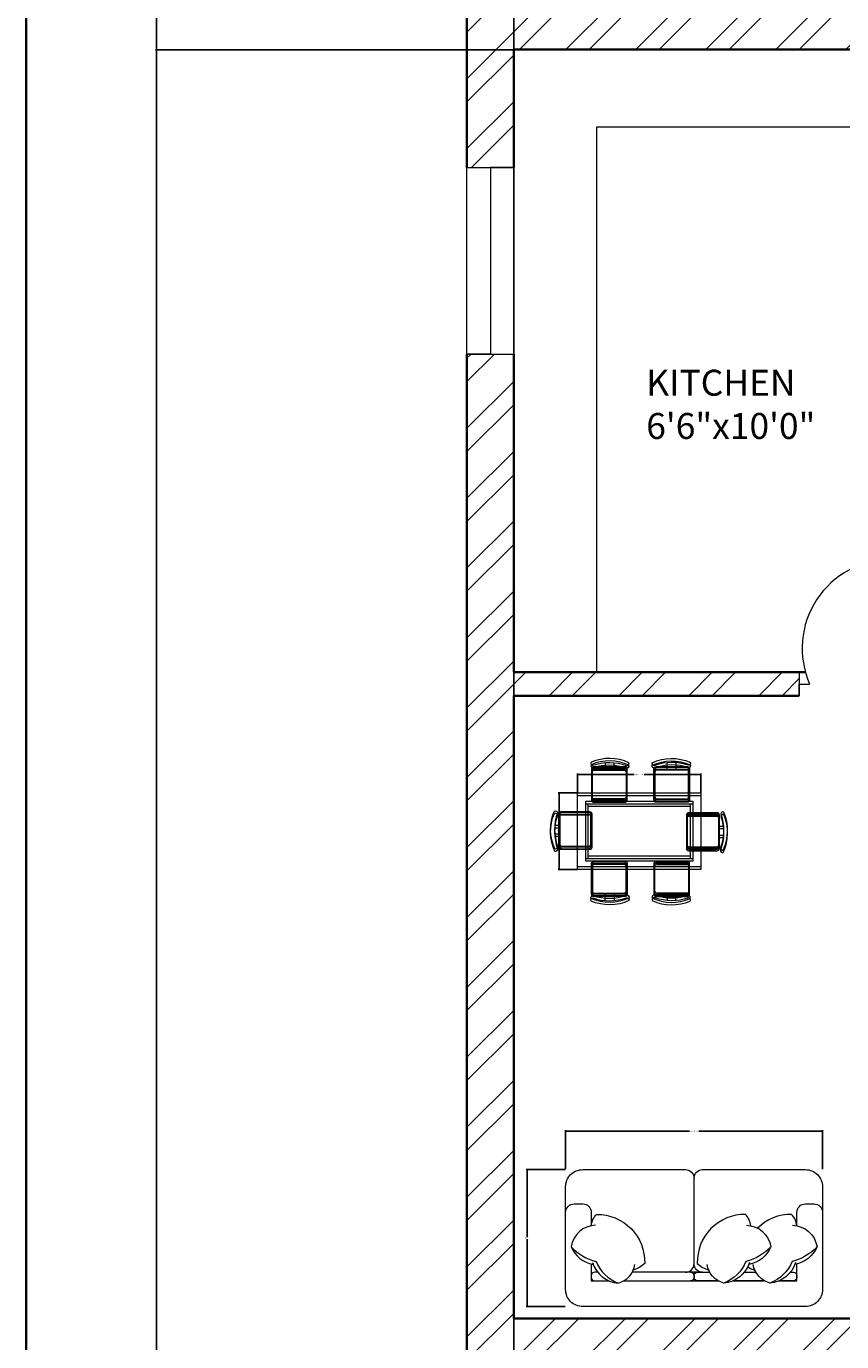
# Model space of a CAD drawing. Units: inches. Extents: x 2552 to 3217, y 1417 to 2737.
# Tile 9 of 25: x 2552 to 2710, y 2138 to 2392. Entities that reach past the tile are written whole.
import ezdxf

# ---------------------------------------------------------------- set-up
doc = ezdxf.new("R2010")
doc.units = ezdxf.units.IN
for name, color, linetype, lineweight in [('A-ANNO-DIMS', 2, 'Continuous', 18), ('A-ANNO-TTLB', 7, 'Continuous', 35), ('A-AREA-IDEN', 7, 'Continuous', 18), ('A-DOOR', 21, 'Continuous', 18), ('A-FLOR-CASE', 9, 'Continuous', 18), ('A-FURN', 8, 'Continuous', 13), ('A-GLAZ', 161, 'Continuous', 18), ('A-WALL', 7, 'Continuous', 35), ('A-WALL-PATT', 217, 'Continuous', 13)]:
    doc.layers.add(name, color=color, linetype=linetype, lineweight=lineweight)
doc.styles.get("Standard").update_dxf_attribs({"font": 'arial.ttf'})
doc.dimstyles.get("Standard").update_dxf_attribs({"dimtxt": 0.18, "dimasz": 0.18, "dimexe": 0.18, "dimexo": 0.0625, "dimgap": 0.09, "dimtad": 0, "dimtih": 1, "dimtoh": 1, "dimdec": 4, "dimzin": 0, "dimdsep": 46, "dimtxsty": 'Standard', "dimcen": 0.09, "dimadec": 0, "dimazin": 0, "dimtfac": 1, "dimtdec": 4, "dimtofl": 0, "dimtmove": 0, "dimatfit": 3, "dimfxl": 1, "dimtolj": 1, "dimtzin": 0, "dimarcsym": 0})

# ---------------------------------------------------------------- blocks, each defined once
blk = doc.blocks.new('TABLE-DINING-RECT')
for points in [[(0, 14.74), (23.77, 14.74), (23.77, 0.48), (0, 0.48)], [(0, 14.74), (23.77, 14.74), (23.77, 0.48), (0, 0.48)], [(0, 14.26), (23.77, 14.26), (23.77, 0), (0, 0)], [(0, 14.26), (23.77, 14.26), (23.77, 0), (0, 0)], [(1.58, 13.15), (22.19, 13.15), (22.19, 2.06), (1.58, 2.06)], [(1.58, 13.15), (22.19, 13.15), (22.19, 2.06), (1.58, 2.06)], [(1.58, 12.68), (22.19, 12.68), (22.19, 1.59), (1.58, 1.59)], [(1.58, 12.68), (22.19, 12.68), (22.19, 1.58), (1.58, 1.58)], [(2.06, 12.68), (21.71, 12.68), (21.71, 2.54), (2.06, 2.54)], [(2.06, 12.68), (21.71, 12.68), (21.71, 2.54), (2.06, 2.54)], [(2.06, 12.2), (21.71, 12.2), (21.71, 2.06), (2.06, 2.06)], [(2.06, 12.2), (21.71, 12.2), (21.71, 2.06), (2.06, 2.06)]]:
    blk.add_lwpolyline(points, close=True)
blk = doc.blocks.new('DINING-CHAIR-NORTH-WEST')
for points in [[(0.39, 7.1, -0.175809), (6.86, 7.05, 0.578392), (7.35, 7.59, 0.214524), (0.05, 7.69, 0.552014), (0.39, 7.1, -0.065079)], [(0.39, 7.1, -0.175809), (6.86, 7.05, 0.578392), (7.35, 7.59, 0.214524), (0.05, 7.69, 0.552014), (0.39, 7.1, -0.065079)], [(0.39, 6.63, -0.175809), (6.86, 6.58, 0.578392), (7.35, 7.12, 0.214524), (0.05, 7.22, 0.552014), (0.39, 6.63, -0.065079)], [(0.39, 6.63, -0.175809), (6.86, 6.58, 0.578392), (7.35, 7.12, 0.214524), (0.05, 7.22, 0.552014), (0.39, 6.63, -0.065079)], [(6.59, 6.84), (0.58, 6.84, 0.414214), (0.16, 6.42), (0.16, 0.9, 0.414214), (0.58, 0.48), (6.59, 0.48, 0.414214), (7.01, 0.9), (7.01, 6.42, 0.414214), (6.59, 6.84)], [(6.59, 6.84), (0.58, 6.84, 0.414214), (0.16, 6.42), (0.16, 0.9, 0.414214), (0.58, 0.48), (6.59, 0.48, 0.414214), (7.01, 0.9), (7.01, 6.42, 0.414214), (6.59, 6.84)], [(6.59, 6.37), (0.58, 6.37, 0.414214), (0.16, 5.95), (0.16, 0.42, 0.414214), (0.58, 0), (6.59, 0, 0.414214), (7.01, 0.42), (7.01, 5.95, 0.414214), (6.59, 6.37)], [(6.59, 6.37), (0.58, 6.37, 0.414214), (0.16, 5.95), (0.16, 0.42, 0.414214), (0.58, 0), (6.59, 0, 0.414214), (7.01, 0.42), (7.01, 5.95, 0.414214), (6.59, 6.37)], [(4.48, 6.84), (4.48, 7.6, -0.064759)], [(4.48, 6.84), (4.48, 7.6, -0.064759)], [(4.48, 6.37), (4.48, 7.13, -0.064759)], [(4.48, 6.37), (4.48, 7.13, -0.064759)]]:
    blk.add_lwpolyline(points, format="xyb")
for points in [[(2.79, 7.62), (2.79, 6.84)], [(2.79, 7.62), (2.79, 6.84)], [(2.79, 7.14), (2.79, 6.37)], [(2.79, 7.14), (2.79, 6.37)]]:
    blk.add_lwpolyline(points)
for points in [[(0.58, 6.65), (6.4, 6.65, -0.414214), (6.82, 6.23), (6.82, 1.09, -0.414214), (6.4, 0.67), (0.58, 0.67, -0.512069), (0.35, 1.09), (0.35, 6.23, -0.512069)], [(0.58, 6.65), (6.4, 6.65, -0.414214), (6.82, 6.23), (6.82, 1.09, -0.414214), (6.4, 0.67), (0.58, 0.67, -0.512069), (0.35, 1.09), (0.35, 6.23, -0.512069)], [(0.58, 6.18), (6.4, 6.18, -0.414214), (6.82, 5.76), (6.82, 0.61, -0.414214), (6.4, 0.19), (0.58, 0.19, -0.512069), (0.35, 0.61), (0.35, 5.76, -0.512069)], [(0.58, 6.18), (6.4, 6.18, -0.414214), (6.82, 5.76), (6.82, 0.61, -0.414214), (6.4, 0.19), (0.58, 0.19, -0.512069), (0.35, 0.61), (0.35, 5.76, -0.512069)]]:
    blk.add_lwpolyline(points, format="xyb", close=True)
blk = doc.blocks.new('SOFA-COMPACT')
at = {"ltscale": 0.03}
blk.add_lwpolyline([(23.09, 26.39, -0.414214), (24.74, 24.74, -0.414214), (26.39, 26.39), (46.19, 26.39, -0.414214), (49.49, 23.09), (49.49, 3.3, -0.414214), (46.19, 0), (3.3, 0, -0.414214), (0, 3.3), (0, 23.09, -0.414214), (3.3, 26.39), (23.09, 26.39, -0.414214), (24.74, 24.74, -0.414214), (26.39, 26.39)], format="xyb", dxfattribs=at)
for points in [[(23.09, 6.6, 0.414214), (24.74, 8.25), (24.74, 24.74, 0.414214)], [(26.39, 6.6, -0.414214), (24.74, 8.25), (24.74, 24.74, -0.414214)], [(0, 18.15, -0.414214), (1.65, 19.79), (3.3, 19.79, -0.414214), (4.95, 18.15), (4.95, 15.59)], [(4.94, 15.59, -0.165541), (5.97, 17.77, -0.425989), (15.23, 8.32, -0.121523), (13.03, 7.02, 7.115464)], [(35.66, 15.59, 0.165541), (34.64, 17.77, 0.425989), (25.37, 8.32, 0.121523), (27.57, 7.02, -7.115464)], [(44.54, 15.59, 0.165541), (43.52, 17.77, 0.200231), (36.97, 15.11, 0.121523)], [(44.54, 15.59), (44.54, 18.15, -0.414214), (46.19, 19.79), (47.84, 19.79, -0.414214), (49.49, 18.15)], [(5.78, 15.69, 0.356772), (1.05, 11.53, 0.249542), (5.33, 8.1, -9.61688)], [(34.82, 15.69, -0.356772), (39.55, 11.53, -0.249542), (35.27, 8.1, 9.61688)], [(43.71, 15.69, -0.356772), (48.44, 11.53, -0.249542), (44.15, 8.1, 9.61688)], [(1.05, 11.53, 0.14773), (5.87, 8.7, 0.213343), (10.12, 4.54, 0.178662)], [(39.55, 11.53, -0.14773), (34.73, 8.7, -0.213343), (30.48, 4.54, -0.178662)], [(48.44, 11.53, -0.14773), (43.62, 8.7, -0.213343), (39.36, 4.54, -0.178662)], [(5.2, 8.47, 0.306663), (10.12, 4.54, 0.30633), (13.34, 8.13, -0.872847)], [(23.09, 6.6, 0.414214), (24.74, 8.25)], [(26.39, 6.6, -0.414214), (24.74, 8.25)], [(35.4, 8.47, -0.306663), (30.48, 4.54, -0.30633), (27.26, 8.13, 0.872847)], [(35.07, 7.66, 0.071865), (36.46, 7.02, -7.115464)], [(44.28, 8.47, -0.306663), (39.36, 4.54, -0.30633), (36.15, 8.13, 0.872847)], [(41.07, 4.95), (44.54, 4.95), (44.54, 8.19, -0.414214)], [(6.21, 6.6), (5.61, 6.6, 0.414214), (4.95, 5.94), (4.95, 5.61, 0.414214), (5.61, 4.95)], [(11.16, 4.95), (24.08, 4.95, 0.414214), (24.74, 5.61), (24.74, 5.94, 0.414214), (24.08, 6.6), (12.82, 6.6, 0.414214)], [(29.44, 4.95), (25.4, 4.95, -0.414214), (24.74, 5.61), (24.74, 5.94, -0.414214), (25.4, 6.6), (27.78, 6.6, -0.414214)], [(34.39, 6.6), (36.66, 6.6, -0.414214)], [(43.28, 6.6), (43.88, 6.6, -0.414214), (44.54, 5.94), (44.54, 5.61, -0.414214), (43.88, 4.95)], [(5.61, 4.95), (8.42, 4.95, 0.414214)], [(38.32, 4.95), (32.18, 4.95, -0.414214)], [(43.88, 4.95), (41.07, 4.95, -0.414214)]]:
    blk.add_lwpolyline(points, format="xyb")
for points in [[(4.95, 8.19), (4.95, 4.95), (8.42, 4.95)], [(11.16, 4.95), (29.44, 4.95)], [(32.18, 4.95), (38.32, 4.95)]]:
    blk.add_lwpolyline(points)
blk.add_lwpolyline([(24.08, 4.95), (25.4, 4.95, -0.414214), (24.74, 5.61), (24.74, 5.94, -0.414214), (25.4, 6.6), (24.08, 6.6, -0.414214), (24.74, 5.94), (24.74, 5.61, -0.414214)], format="xyb", close=True)
blk = doc.blocks.new('WIN-36')
for p, q in [((4.5, 36), (0, 36)), ((0, 36), (9, 36)), ((0, 36), (0, 0)), ((4.5, 0), (4.5, 36)), ((9, 36), (9, 0)), ((0, 0), (9, 0)), ((9, 0), (4.5, 0))]:
    blk.add_line(p, q)
blk = doc.blocks.new('*D23')
at = {"layer": 'A-ANNO-DIMS', "color": 0, "lineweight": -2, "transparency": 16777216}
for p, q in [((2658.65, 2243.82), (2658.65, 2247.5)), ((2658.83, 2247.32), (2669.57, 2247.32)), ((2682.24, 2247.32), (2671.5, 2247.32)), ((2682.42, 2243.82), (2682.42, 2247.5))]:
    blk.add_line(p, q, dxfattribs=at)
at = {"layer": 'A-ANNO-DIMS', "color": 0, "transparency": 16777216}
for points in [[(2658.83, 2247.35), (2658.83, 2247.29), (2658.65, 2247.32)], [(2682.24, 2247.35), (2682.24, 2247.29), (2682.42, 2247.32)]]:
    blk.add_solid(points, dxfattribs=at)
at = {"layer": 'Defpoints', "color": 0, "transparency": 16777216}
for p in [(2682.42, 2247.32), (2658.65, 2243.76), (2682.42, 2243.76)]:
    blk.add_point(p, dxfattribs=at)
at = {"layer": 'A-ANNO-DIMS', "color": 0, "transparency": 16777216, "insert": (2670.54, 2247.32), "char_height": 0.18, "attachment_point": 5}
blk.add_mtext('\\A1;TABLE 24 TYP.', dxfattribs=at)
blk = doc.blocks.new('*D24')
at = {"layer": 'A-ANNO-DIMS', "color": 0, "lineweight": -2, "transparency": 16777216}
for p, q in [((2658.59, 2243.76), (2654.91, 2243.76)), ((2655.09, 2243.58), (2655.09, 2236.57)), ((2655.09, 2229.2), (2655.09, 2236.2)), ((2658.59, 2229.02), (2654.91, 2229.02))]:
    blk.add_line(p, q, dxfattribs=at)
at = {"layer": 'A-ANNO-DIMS', "color": 0, "transparency": 16777216}
for points in [[(2655.06, 2243.58), (2655.12, 2243.58), (2655.09, 2243.76)], [(2655.06, 2229.2), (2655.12, 2229.2), (2655.09, 2229.02)]]:
    blk.add_solid(points, dxfattribs=at)
at = {"layer": 'Defpoints', "color": 0, "transparency": 16777216}
for p in [(2655.09, 2243.76), (2658.65, 2243.76), (2658.65, 2229.02)]:
    blk.add_point(p, dxfattribs=at)
at = {"layer": 'A-ANNO-DIMS', "color": 0, "transparency": 16777216, "insert": (2655.09, 2236.39), "char_height": 0.18, "attachment_point": 5}
blk.add_mtext('\\A1;15 TYP.', dxfattribs=at)
blk = doc.blocks.new('*D43')
at = {"layer": 'A-ANNO-DIMS', "color": 0, "lineweight": -2, "transparency": 16777216}
for p, q in [((2656.35, 2171.24), (2656.35, 2178.78)), ((2656.53, 2178.6), (2680.19, 2178.6)), ((2705.66, 2178.6), (2682, 2178.6)), ((2705.84, 2171.24), (2705.84, 2178.78))]:
    blk.add_line(p, q, dxfattribs=at)
at = {"layer": 'A-ANNO-DIMS', "color": 0, "transparency": 16777216}
for points in [[(2656.53, 2178.63), (2656.53, 2178.57), (2656.35, 2178.6)], [(2705.66, 2178.63), (2705.66, 2178.57), (2705.84, 2178.6)]]:
    blk.add_solid(points, dxfattribs=at)
at = {"layer": 'Defpoints', "color": 0, "transparency": 16777216}
for p in [(2705.84, 2178.6), (2656.35, 2171.17), (2705.84, 2171.17)]:
    blk.add_point(p, dxfattribs=at)
at = {"layer": 'A-ANNO-DIMS', "color": 0, "transparency": 16777216, "insert": (2681.1, 2178.6), "char_height": 0.18, "attachment_point": 5}
blk.add_mtext('\\A1;SOFA 49 TYP.', dxfattribs=at)
blk = doc.blocks.new('*D44')
at = {"layer": 'A-ANNO-DIMS', "color": 0, "lineweight": -2, "transparency": 16777216}
for p, q in [((2656.29, 2171.17), (2648.75, 2171.17)), ((2648.93, 2170.99), (2648.93, 2158.16)), ((2648.93, 2144.96), (2648.93, 2157.79)), ((2656.29, 2144.78), (2648.75, 2144.78))]:
    blk.add_line(p, q, dxfattribs=at)
at = {"layer": 'A-ANNO-DIMS', "color": 0, "transparency": 16777216}
for points in [[(2648.9, 2170.99), (2648.96, 2170.99), (2648.93, 2171.17)], [(2648.9, 2144.96), (2648.96, 2144.96), (2648.93, 2144.78)]]:
    blk.add_solid(points, dxfattribs=at)
at = {"layer": 'Defpoints', "color": 0, "transparency": 16777216}
for p in [(2648.93, 2171.17), (2656.35, 2171.17), (2656.35, 2144.78)]:
    blk.add_point(p, dxfattribs=at)
at = {"layer": 'A-ANNO-DIMS', "color": 0, "transparency": 16777216, "insert": (2648.93, 2157.98), "char_height": 0.18, "attachment_point": 5}
blk.add_mtext('\\A1;26 TYP.', dxfattribs=at)
blk = doc.blocks.new('*D50')
at = {"layer": 'A-ANNO-DIMS', "color": 0, "lineweight": -2, "transparency": 16777216}
for p, q in [((2637.29, 2649.51), (2577.37, 2649.51)), ((2577.55, 2649.33), (2577.55, 2096.19)), ((2577.55, 1542.69), (2577.55, 2095.83)), ((2637.29, 1542.51), (2577.37, 1542.51))]:
    blk.add_line(p, q, dxfattribs=at)
at = {"layer": 'A-ANNO-DIMS', "color": 0, "transparency": 16777216}
for points in [[(2577.52, 2649.33), (2577.58, 2649.33), (2577.55, 2649.51)], [(2577.52, 1542.69), (2577.58, 1542.69), (2577.55, 1542.51)]]:
    blk.add_solid(points, dxfattribs=at)
at = {"layer": 'Defpoints', "color": 0, "transparency": 16777216}
for p in [(2577.55, 2649.51), (2637.35, 2649.51), (2637.35, 1542.51)]:
    blk.add_point(p, dxfattribs=at)
at = {"layer": 'A-ANNO-DIMS', "color": 0, "transparency": 16777216, "insert": (2577.55, 2096.01), "char_height": 0.18, "attachment_point": 5}
blk.add_mtext('\\A1;1107', dxfattribs=at)
blk = doc.blocks.new('*D64')
at = {"layer": 'A-ANNO-DIMS', "color": 0, "lineweight": -2, "transparency": 16777216}
for p, q in [((2646.35, 1551.58), (2646.35, 2709.49)), ((2646.53, 2709.31), (2802.77, 2709.31)), ((2959.93, 2709.31), (2803.69, 2709.31)), ((2960.11, 1551.58), (2960.11, 2709.49))]:
    blk.add_line(p, q, dxfattribs=at)
at = {"layer": 'A-ANNO-DIMS', "color": 0, "transparency": 16777216}
for points in [[(2646.53, 2709.34), (2646.53, 2709.28), (2646.35, 2709.31)], [(2959.93, 2709.34), (2959.93, 2709.28), (2960.11, 2709.31)]]:
    blk.add_solid(points, dxfattribs=at)
at = {"layer": 'Defpoints', "color": 0, "transparency": 16777216}
for p in [(2960.11, 2709.31), (2646.35, 1551.51), (2960.11, 1551.51)]:
    blk.add_point(p, dxfattribs=at)
at = {"layer": 'A-ANNO-DIMS', "color": 0, "transparency": 16777216, "insert": (2803.23, 2709.31), "char_height": 0.18, "attachment_point": 5}
blk.add_mtext('\\A1;313.76', dxfattribs=at)
blk = doc.blocks.new('*D69')
at = {"layer": 'A-ANNO-DIMS', "color": 0, "lineweight": -2, "transparency": 16777216}
for p, q in [((2908.79, 2403.41), (2577.37, 2403.41)), ((2577.55, 2403.23), (2577.55, 2395.39)), ((2577.55, 2387.19), (2577.55, 2395.03)), ((2917.79, 2387.01), (2577.37, 2387.01))]:
    blk.add_line(p, q, dxfattribs=at)
at = {"layer": 'A-ANNO-DIMS', "color": 0, "transparency": 16777216}
for points in [[(2577.52, 2403.23), (2577.58, 2403.23), (2577.55, 2403.41)], [(2577.52, 2387.19), (2577.58, 2387.19), (2577.55, 2387.01)]]:
    blk.add_solid(points, dxfattribs=at)
at = {"layer": 'Defpoints', "color": 0, "transparency": 16777216}
for p in [(2577.55, 2403.41), (2908.85, 2403.41), (2917.85, 2387.01)]:
    blk.add_point(p, dxfattribs=at)
at = {"layer": 'A-ANNO-DIMS', "color": 0, "transparency": 16777216, "insert": (2577.55, 2395.21), "char_height": 0.18, "attachment_point": 5}
blk.add_mtext('\\A1;16.4', dxfattribs=at)

msp = doc.modelspace()

# ---------------------------------------------------------------- hatches: boundary and pattern name
at = {"layer": 'A-WALL-PATT'}
h = msp.add_hatch(dxfattribs=at)
h.set_pattern_fill('ANSI32', color=256)
h.paths.add_polyline_path([(2756.676, 2649.5125), (2637.3535, 2649.5125), (2637.3535, 2617.9626), (2641.8535, 2617.9626), (2646.3535, 2617.9626), (2646.3535, 2640.5125), (2724.3535, 2640.5125), (2724.3535, 2520.5125), (2720.299, 2520.5125), (2720.299, 2516.0125), (2733.4075, 2516.0125), (2733.4075, 2518.2213), (2733.4075, 2520.5125), (2728.8535, 2520.5125), (2728.8535, 2640.5125), (2756.676, 2640.5125)])
h.paths.add_polyline_path([(2848.8535, 2649.5125), (2804.676, 2649.5125), (2804.676, 2640.5125), (2839.8535, 2640.5125), (2839.8535, 2598.3517), (2848.8535, 2598.3517)])
h.paths.add_polyline_path([(2646.3535, 2516.0125), (2697.9593, 2516.0125), (2697.9593, 2518.2625), (2697.9593, 2520.5125), (2646.3535, 2520.5125), (2646.3535, 2581.9626), (2637.3535, 2581.9626), (2637.3535, 2364.3298), (2646.3535, 2364.3298), (2646.3535, 2387.0125), (2724.3535, 2387.0125), (2724.3535, 2267.0125), (2721.0443, 2267.0125), (2721.0443, 2262.5125), (2733.7854, 2262.5125), (2733.7854, 2264.7625), (2733.7854, 2267.0125), (2728.8535, 2267.0125), (2728.8535, 2387.0125), (2839.8535, 2387.0125), (2839.8535, 2363.8387), (2848.8535, 2363.8387), (2848.8535, 2403.7415), (2844.3535, 2403.7415), (2839.8535, 2403.7415), (2839.8535, 2396.0125), (2646.3535, 2396.0125)])
h.paths.add_polyline_path([(2848.8535, 2550.3517), (2844.3535, 2550.3517), (2839.8535, 2550.3517), (2839.8535, 2520.5125), (2801.9195, 2520.5125), (2801.9195, 2518.2625), (2801.9195, 2516.0125), (2839.8535, 2516.0125), (2839.8535, 2507.5813), (2848.8535, 2507.5813)], flags=17)
h.paths.add_polyline_path([(2848.8535, 2483.5813), (2844.3535, 2483.5813), (2839.8535, 2483.5813), (2839.8535, 2468.0125), (2773.8535, 2468.0125), (2773.8535, 2516.0125), (2778.1336, 2516.0125), (2778.1336, 2520.5125), (2766.696, 2520.5125), (2766.696, 2518.2625), (2766.696, 2516.0125), (2769.3535, 2516.0125), (2769.3535, 2463.5125), (2839.8535, 2463.5125), (2839.8535, 2431.0782), (2848.8535, 2431.0782)], flags=17)
h.paths.add_polyline_path([(2917.8535, 2569.2764), (2913.3535, 2569.2764), (2908.8535, 2569.2764), (2908.8535, 2433.001), (2917.8535, 2433.001), (2917.8535, 2516.0125), (2967.486, 2516.0125), (2967.486, 2520.5125), (2917.8535, 2520.5125)])
h.paths.add_polyline_path([(3000.3535, 2640.5125), (2995.8535, 2640.5125), (2995.8535, 2520.5125), (2990.688, 2520.5125), (2990.688, 2516.0125), (3004.0844, 2516.0125), (3004.0844, 2518.2625), (3004.0844, 2520.5125), (3000.3535, 2520.5125)])
h.paths.add_polyline_path([(3120.3535, 2561.3689), (3115.8535, 2561.3689), (3111.3535, 2561.3689), (3111.3535, 2520.5125), (3070.9814, 2520.5125), (3070.9814, 2518.2625), (3070.9814, 2516.0125), (3111.3535, 2516.0125), (3111.3535, 2505.1841), (3120.3535, 2505.1841)])
h.paths.add_polyline_path([(3120.3535, 2481.1841), (3115.8535, 2481.1841), (3111.3535, 2481.1841), (3111.3535, 2468.0125), (3045.3535, 2468.0125), (3045.3535, 2516.0125), (3048.9787, 2516.0125), (3048.9787, 2520.5125), (3036.3395, 2520.5125), (3036.3395, 2516.0125), (3040.8535, 2516.0125), (3040.8535, 2463.5125), (3111.3535, 2463.5125), (3111.3535, 2396.0125), (2917.8535, 2396.0125), (2917.8535, 2403.4124), (2913.3535, 2403.4124), (2908.8535, 2403.4124), (2908.8535, 2182.5756), (2917.8535, 2182.5756), (2917.8535, 2262.5125), (2968.001, 2262.5125), (2968.001, 2264.7625), (2968.001, 2267.0125), (2917.8535, 2267.0125), (2917.8535, 2387.0125), (3111.3535, 2387.0125), (3111.3535, 2352.2435), (3120.3535, 2352.2435)])
h.paths.add_polyline_path([(3120.3535, 2304.2435), (3115.8535, 2304.2435), (3111.3535, 2304.2435), (3111.3535, 2267.0125), (3073.8616, 2267.0125), (3073.8616, 2264.7625), (3073.8616, 2262.5125), (3111.3535, 2262.5125), (3111.3535, 2252.376), (3120.3535, 2252.376)], flags=17)
h.paths.add_polyline_path([(3120.3535, 2228.376), (3115.8535, 2228.376), (3111.3535, 2228.376), (3111.3535, 2214.5125), (3045.3535, 2214.5125), (3045.3535, 2262.5125), (3049.3096, 2262.5125), (3049.3096, 2267.0125), (3035.0125, 2267.0125), (3035.0125, 2262.5125), (3040.8535, 2262.5125), (3040.8535, 2210.0125), (3111.3535, 2210.0125), (3111.3535, 2142.5125), (2917.8535, 2142.5125), (2917.8535, 2150.2408), (2913.3535, 2150.2408), (2908.8535, 2150.2408), (2908.8535, 1924.9905), (2917.8535, 1924.9905), (2917.8535, 2009.0125), (2971.959, 2009.0125), (2971.959, 2011.2625), (2971.959, 2013.5125), (2917.8535, 2013.5125), (2917.8535, 2133.5125), (2995.8535, 2133.5125), (2995.8535, 2013.5125), (2992.1797, 2013.5125), (2992.1797, 2009.0125), (3004.3344, 2009.0125), (3004.3344, 2011.2625), (3004.3344, 2013.5125), (3000.3535, 2013.5125), (3000.3535, 2133.5125), (3111.3535, 2133.5125), (3111.3535, 2115.0291), (3120.3535, 2115.0291)])
h.paths.add_polyline_path([(3000.3535, 2387.0125), (2995.8535, 2387.0125), (2995.8535, 2267.0125), (2991.3326, 2267.0125), (2991.3326, 2262.5125), (3004.1044, 2262.5125), (3004.1044, 2264.7625), (3004.1044, 2267.0125), (3000.3535, 2267.0125)], flags=17)
h.paths.add_polyline_path([(3120.3535, 1973.2388), (3115.8535, 1973.2388), (3111.3535, 1973.2388), (3111.3535, 1961.0125), (3045.3535, 1961.0125), (3045.3535, 2009.0125), (3048.9101, 2009.0125), (3048.9101, 2013.5125), (3037.105, 2013.5125), (3037.105, 2011.2625), (3037.105, 2009.0125), (3040.8535, 2009.0125), (3040.8535, 1956.5125), (3111.3535, 1956.5125), (3111.3535, 1889.0125), (2917.8535, 1889.0125), (2917.8535, 1895.7215), (2913.3535, 1895.7215), (2908.8535, 1895.7215), (2908.8535, 1844.2217), (2917.8535, 1844.2217), (2917.8535, 1880.0125), (3111.3535, 1880.0125), (3111.3535, 1846.9541), (3120.3535, 1846.9541)])
h.paths.add_polyline_path([(3120.3535, 2067.0291), (3111.3535, 2067.0291), (3111.3535, 2013.5125), (3071.3001, 2013.5125), (3071.3001, 2009.0125), (3111.3535, 2009.0125), (3111.3535, 1997.2388), (3120.3535, 1997.2388)], flags=0)
h.paths.add_polyline_path([(3120.3535, 1798.9541), (3115.8535, 1798.9541), (3111.3535, 1798.9541), (3111.3535, 1760.0125), (3071.2497, 1760.0125), (3071.2497, 1757.7625), (3071.2497, 1755.5125), (3111.3535, 1755.5125), (3111.3535, 1746.162), (3120.3535, 1746.2478)])
h.paths.add_polyline_path([(3120.3535, 1722.2049), (3111.3535, 1722.2049), (3111.3535, 1707.5125), (3045.3535, 1707.5125), (3045.3535, 1755.5125), (3048.6624, 1755.5125), (3048.6624, 1760.0125), (3035.3703, 1760.0125), (3035.3703, 1755.5125), (3040.8535, 1755.5125), (3040.8535, 1703.0125), (3111.3535, 1703.0125), (3111.3535, 1635.5125), (2917.8535, 1635.5125), (2917.8535, 1643.1366), (2913.3535, 1643.1366), (2908.8535, 1643.1366), (2908.8535, 1626.5125), (3120.3535, 1626.5125)])
h.paths.add_polyline_path([(2917.8535, 1755.5125), (2973.2287, 1755.5125), (2973.2287, 1757.7625), (2973.2287, 1760.0125), (2917.8535, 1760.0125), (2917.8535, 1808.2217), (2913.3535, 1808.2217), (2908.8535, 1808.2217), (2908.8535, 1676.1665), (2917.8535, 1676.1665)])
h.paths.add_polyline_path([(3000.3535, 1880.0125), (2995.8535, 1880.0125), (2995.8535, 1760.0125), (2992.9329, 1760.0125), (2992.9329, 1755.5125), (3003.8766, 1755.5125), (3003.8766, 1757.7625), (3003.8766, 1760.0125), (3000.3535, 1760.0125)])
h.paths.add_polyline_path([(2848.8535, 1896.6971), (2844.3535, 1896.6971), (2839.8535, 1896.6971), (2839.8535, 1889.0125), (2646.3535, 1889.0125), (2646.3535, 2009.0125), (2700.5253, 2009.0125), (2700.5253, 2011.2625), (2700.5253, 2013.5125), (2646.3535, 2013.5125), (2646.3535, 2053.1812), (2641.8535, 2053.1812), (2637.3535, 2053.1812), (2637.3535, 1836.254), (2646.3535, 1836.254), (2646.3535, 1880.0125), (2724.3535, 1880.0125), (2724.3535, 1760.0125), (2721.2473, 1760.0125), (2721.2473, 1755.5125), (2731.9187, 1755.5125), (2731.9187, 1757.7625), (2731.9187, 1760.0125), (2728.8535, 1760.0125), (2728.8535, 1880.0125), (2839.8535, 1880.0125), (2839.8535, 1840.3813), (2848.8535, 1840.3813)])
h.paths.add_polyline_path([(2848.8535, 1792.3813), (2844.3535, 1792.3813), (2839.8535, 1792.3813), (2839.8535, 1760.0125), (2797.8845, 1760.0125), (2797.8845, 1755.5125), (2839.8535, 1755.5125), (2839.8535, 1743.3688), (2844.3535, 1743.3688), (2848.8535, 1743.3688)], flags=0)
h.paths.add_polyline_path([(2848.8535, 1719.3688), (2844.3535, 1719.3688), (2839.8535, 1719.3688), (2839.8535, 1707.5125), (2773.8535, 1707.5125), (2773.8535, 1755.5125), (2777.716, 1755.5125), (2777.716, 1760.0125), (2760.9247, 1760.0125), (2760.9247, 1757.9721), (2760.9247, 1755.5125), (2769.3535, 1755.5125), (2769.3535, 1703.0125), (2839.8535, 1703.0125), (2839.8535, 1673.0277), (2848.8535, 1672.9407)], flags=0)
h.paths.add_polyline_path([(2646.3535, 1755.5125), (2702.9171, 1755.5125), (2702.9171, 1757.7625), (2702.9171, 1760.0125), (2646.3535, 1760.0125), (2646.3535, 1800.254), (2641.8535, 1800.254), (2637.3535, 1800.254), (2637.3535, 1626.5125), (2848.8535, 1626.5125), (2848.8535, 1643.1187), (2844.3535, 1643.1187), (2839.8535, 1643.1187), (2839.8535, 1635.5125), (2646.3535, 1635.5125)])
h.paths.add_polyline_path([(2848.8535, 2148.8427), (2844.3535, 2148.8427), (2839.8535, 2148.8427), (2839.8535, 2142.5125), (2646.3535, 2142.5125), (2646.3535, 2262.5125), (2701.3562, 2262.5125), (2701.3562, 2264.7625), (2701.3562, 2267.0125), (2646.3535, 2267.0125), (2646.3535, 2328.3298), (2637.3535, 2328.3298), (2637.3535, 2089.1812), (2646.3535, 2089.1812), (2646.3535, 2133.5125), (2839.8535, 2133.5125), (2839.8535, 2097.5966), (2848.8535, 2097.5966)])
h.paths.add_polyline_path([(2728.8535, 2133.5125), (2724.3535, 2133.5125), (2724.3535, 2013.5125), (2719.6039, 2013.5125), (2719.6039, 2009.0125), (2732.5784, 2009.0125), (2732.5784, 2011.2625), (2732.5784, 2013.5125), (2728.8535, 2013.5125)])
h.paths.add_polyline_path([(2848.8535, 1970.0557), (2844.3535, 1970.0557), (2839.8535, 1970.0557), (2839.8535, 1961.0125), (2773.8535, 1961.0125), (2773.8535, 2009.0125), (2777.3388, 2009.0125), (2777.3388, 2013.5125), (2764.7681, 2013.5125), (2764.7681, 2009.0125), (2769.3535, 2009.0125), (2769.3535, 1956.5125), (2839.8535, 1956.5125), (2839.8535, 1924.7199), (2848.8535, 1924.7199)], flags=17)
h.paths.add_polyline_path([(2848.8535, 2049.5966), (2844.3535, 2049.5966), (2839.8535, 2049.5966), (2839.8535, 2013.5125), (2798.198, 2013.5125), (2798.198, 2011.2625), (2798.198, 2009.0125), (2839.8535, 2009.0125), (2839.8535, 1994.0557), (2848.8535, 1994.0557)], flags=17)
h.paths.add_polyline_path([(2848.8535, 2315.8387), (2839.8535, 2315.8387), (2839.8535, 2267.0125), (2799.3375, 2267.0125), (2799.3375, 2264.7625), (2799.3375, 2262.5125), (2839.8535, 2262.5125), (2839.8535, 2253.2843), (2848.8535, 2253.2843)], flags=17)
h.paths.add_polyline_path([(2848.8535, 2229.2843), (2839.8535, 2229.2843), (2839.8535, 2177.6936), (2848.8535, 2177.6936)], flags=17)
h.paths.add_polyline_path([(2839.8535, 2214.5125), (2773.8535, 2214.5125), (2773.8535, 2262.5125), (2777.6984, 2262.5125), (2777.6984, 2267.0125), (2763.8226, 2267.0125), (2763.8226, 2262.5125), (2769.3535, 2262.5125), (2769.3535, 2210.0125), (2839.8535, 2210.0125)], flags=17)
h.paths.add_polyline_path([(3050.32, 2520.2817), (3088.9114, 2520.2817), (3088.9114, 2538.939), (3050.32, 2538.939)], flags=9)

# ---------------------------------------------------------------- linework, layer by layer
at = {"layer": 'A-ANNO-TTLB'}
msp.add_lwpolyline([(2552.473, 2736.5692), (3216.7862, 2736.5692), (3216.7862, 1416.6914), (2552.473, 1416.6914)], close=True, dxfattribs=at)
at = {"layer": 'A-DOOR'}
for p, q in [((2701.3562, 2267.0125), (2701.3562, 2262.5125)), ((2701.3562, 2262.5125), (2701.3562, 2264.7625)), ((2701.3562, 2264.7625), (2703.3562, 2264.7625))]:
    msp.add_line(p, q, dxfattribs=at)
msp.add_arc((2719.0443, 2271.6351), 17.1274, 90, 203.657264, dxfattribs=at)
at = {"layer": 'A-FLOR-CASE'}
for p, q in [((2662.3425, 2267.0125), (2662.3425, 2372.1585)), ((2662.3425, 2372.1585), (2724.3535, 2372.1585))]:
    msp.add_line(p, q, dxfattribs=at)
at = {"layer": 'A-FURN'}
for points in [[(2673.5175, 2249.0427, -0.57839206), (2673.027, 2249.5821, -0.21452438), (2680.3353, 2249.6801, -0.55201397), (2679.9919, 2249.0918, 0.1758092), (2673.5175, 2249.0427)], [(2673.5175, 2249.0425, -0.57839206), (2673.027, 2249.5818, -0.21452438), (2680.3353, 2249.6799, -0.55201397), (2679.992, 2249.0915, 0.1758092), (2673.5175, 2249.0425)], [(2673.5175, 2248.5673, -0.57839206), (2673.027, 2249.1067, -0.21452438), (2680.3353, 2249.2047, -0.55201397), (2679.9919, 2248.6164, 0.1758092), (2673.5175, 2248.5673)], [(2673.5175, 2248.5671, -0.57839206), (2673.027, 2249.1064, -0.21452438), (2680.3353, 2249.2045, -0.55201397), (2679.992, 2248.6161, 0.1758092), (2673.5175, 2248.5671)], [(2679.8028, 2248.8319, -0.41421356), (2680.2234, 2248.4114), (2680.2234, 2242.8847, -0.41421356), (2679.8028, 2242.4642), (2673.7922, 2242.4642, -0.41421356), (2673.3717, 2242.8847), (2673.3717, 2248.4114, -0.41421356), (2673.7922, 2248.8319), (2679.8028, 2248.8319)], [(2679.8029, 2248.8317, -0.41421356), (2680.2234, 2248.4112), (2680.2234, 2242.8845, -0.41421356), (2679.8029, 2242.464), (2673.7922, 2242.464, -0.41421356), (2673.3717, 2242.8845), (2673.3717, 2248.4112, -0.41421356), (2673.7922, 2248.8317), (2679.8029, 2248.8317)], [(2675.9034, 2248.8319), (2675.9034, 2249.5921, 0.06475861)], [(2675.9034, 2248.8317), (2675.9034, 2249.5918, 0.06475861)], [(2675.9034, 2248.3565), (2675.9034, 2249.1167, 0.06475861)], [(2675.9034, 2248.3563), (2675.9034, 2249.1164, 0.06475861)], [(2679.8028, 2248.3565, -0.41421356), (2680.2234, 2247.936), (2680.2234, 2242.4093, -0.41421356), (2679.8028, 2241.9888), (2673.7922, 2241.9888, -0.41421356), (2673.3717, 2242.4093), (2673.3717, 2247.936, -0.41421356), (2673.7922, 2248.3565), (2679.8028, 2248.3565)], [(2679.8029, 2248.3563, -0.41421356), (2680.2234, 2247.9357), (2680.2234, 2242.4091, -0.41421356), (2679.8029, 2241.9885), (2673.7922, 2241.9885, -0.41421356), (2673.3717, 2242.4091), (2673.3717, 2247.9357, -0.41421356), (2673.7922, 2248.3563), (2679.8029, 2248.3563)], [(2654.8189, 2233.457, -0.57839206), (2654.2795, 2232.9665, -0.21452438), (2654.1815, 2240.2747, -0.55201397), (2654.7698, 2239.9314, 0.17580937), (2654.8189, 2233.457)], [(2654.8189, 2233.4567, -0.57839206), (2654.2796, 2232.9662, -0.21452438), (2654.1815, 2240.2745, -0.55201397), (2654.7699, 2239.9312, 0.17580937), (2654.8189, 2233.4567)], [(2654.8189, 2232.9815, -0.57839206), (2654.2795, 2232.491, -0.21452438), (2654.1815, 2239.7993, -0.55201397), (2654.7698, 2239.456, 0.17580937), (2654.8189, 2232.9815)], [(2654.8189, 2232.9813, -0.57839206), (2654.2796, 2232.4908, -0.21452438), (2654.1815, 2239.7991, -0.55201397), (2654.7699, 2239.4557, 0.17580937), (2654.8189, 2232.9813)], [(2655.0297, 2239.7423, -0.41421356), (2655.4502, 2240.1628), (2660.9769, 2240.1628, -0.41421356), (2661.3974, 2239.7423), (2661.3974, 2233.7316, -0.41421356), (2660.9769, 2233.3111), (2655.4502, 2233.3111, -0.41421356), (2655.0297, 2233.7316), (2655.0297, 2239.7423)], [(2655.0297, 2239.742, -0.41421356), (2655.4502, 2240.1626), (2660.9769, 2240.1626, -0.41421356), (2661.3974, 2239.742), (2661.3974, 2233.7314, -0.41421356), (2660.9769, 2233.3109), (2655.4502, 2233.3109, -0.41421356), (2655.0297, 2233.7314), (2655.0297, 2239.742)], [(2655.0297, 2239.2669, -0.41421356), (2655.4502, 2239.6874), (2660.9769, 2239.6874, -0.41421356), (2661.3974, 2239.2669), (2661.3974, 2233.2562, -0.41421356), (2660.9769, 2232.8357), (2655.4502, 2232.8357, -0.41421356), (2655.0297, 2233.2562), (2655.0297, 2239.2669)], [(2655.0297, 2239.2666, -0.41421356), (2655.4502, 2239.6871), (2660.9769, 2239.6871, -0.41421356), (2661.3974, 2239.2666), (2661.3974, 2233.256, -0.41421356), (2660.9769, 2232.8355), (2655.4502, 2232.8355, -0.41421356), (2655.0297, 2233.256), (2655.0297, 2239.2666)], [(2685.9818, 2239.5364, 0.41421356), (2685.5613, 2239.957), (2680.0346, 2239.957, 0.41421356), (2679.6141, 2239.5364), (2679.6141, 2233.5258, 0.41421356), (2680.0346, 2233.1053), (2685.5613, 2233.1053, 0.41421356), (2685.9818, 2233.5258), (2685.9818, 2239.5364)], [(2685.9818, 2239.5362, 0.41421356), (2685.5613, 2239.9567), (2680.0346, 2239.9567, 0.41421356), (2679.6141, 2239.5362), (2679.6141, 2233.5255, 0.41421356), (2680.0346, 2233.105), (2685.5613, 2233.105, 0.41421356), (2685.9818, 2233.5255), (2685.9818, 2239.5362)], [(2685.9818, 2239.061, 0.41421356), (2685.5613, 2239.4815), (2680.0346, 2239.4815, 0.41421356), (2679.6141, 2239.061), (2679.6141, 2233.0504, 0.41421356), (2680.0346, 2232.6299), (2685.5613, 2232.6299, 0.41421356), (2685.9818, 2233.0504), (2685.9818, 2239.061)], [(2685.9818, 2239.0608, 0.41421356), (2685.5613, 2239.4813), (2680.0346, 2239.4813, 0.41421356), (2679.6141, 2239.0608), (2679.6141, 2233.0501, 0.41421356), (2680.0346, 2232.6296), (2685.5613, 2232.6296, 0.41421356), (2685.9818, 2233.0501), (2685.9818, 2239.0608)], [(2686.2416, 2239.7255, -0.17580919), (2686.1926, 2233.2511, 0.57839206), (2686.7319, 2232.7606, 0.21452438), (2686.83, 2240.0689, 0.55201397), (2686.2416, 2239.7256, -0.06507904)], [(2686.2416, 2239.2501, -0.17580919), (2686.1926, 2232.7757, 0.57839206), (2686.7319, 2232.2852, 0.21452438), (2686.83, 2239.5935, 0.55201397), (2686.2416, 2239.2501, -0.06507904)], [(2686.2417, 2239.7253, -0.17580919), (2686.1926, 2233.2509, 0.57839206), (2686.732, 2232.7604, 0.21452438), (2686.83, 2240.0686, 0.55201397), (2686.2417, 2239.7253, -0.06507904)], [(2686.2417, 2239.2499, -0.17580919), (2686.1926, 2232.7754, 0.57839206), (2686.732, 2232.2849, 0.21452438), (2686.83, 2239.5932, 0.55201397), (2686.2417, 2239.2499, -0.06507904)], [(2655.0297, 2235.8429), (2654.2695, 2235.8429, 0.06475861)], [(2655.0297, 2235.8426), (2654.2695, 2235.8426, 0.06475861)], [(2655.0297, 2235.3675), (2654.2695, 2235.3675, 0.06475861)], [(2655.0297, 2235.3672), (2654.2695, 2235.3672, 0.06475861)], [(2685.9818, 2235.637), (2686.742, 2235.637, -0.06475861)], [(2685.9818, 2235.6368), (2686.742, 2235.6368, -0.06475861)], [(2685.9818, 2235.1616), (2686.742, 2235.1616, -0.06475861)], [(2685.9818, 2235.1614), (2686.742, 2235.1614, -0.06475861)], [(2667.7922, 2224.2644), (2661.7815, 2224.2644, -0.41421356), (2661.361, 2224.6849), (2661.361, 2230.2116, -0.41421356), (2661.7815, 2230.6322), (2667.7922, 2230.6322, -0.41421356), (2668.2127, 2230.2116), (2668.2127, 2224.6849, -0.41421356), (2667.7922, 2224.2644)], [(2667.7922, 2224.2642), (2661.7815, 2224.2642, -0.41421356), (2661.361, 2224.6847), (2661.361, 2230.2114, -0.41421356), (2661.7815, 2230.6319), (2667.7922, 2230.6319, -0.41421356), (2668.2127, 2230.2114), (2668.2127, 2224.6847, -0.41421356), (2667.7922, 2224.2642)], [(2667.7922, 2223.789), (2661.7815, 2223.789, -0.41421356), (2661.361, 2224.2095), (2661.361, 2229.7362, -0.41421356), (2661.7815, 2230.1567), (2667.7922, 2230.1567, -0.41421356), (2668.2127, 2229.7362), (2668.2127, 2224.2095, -0.41421356), (2667.7922, 2223.789)], [(2667.7922, 2223.7888), (2661.7815, 2223.7888, -0.41421356), (2661.361, 2224.2093), (2661.361, 2229.736, -0.41421356), (2661.7815, 2230.1565), (2667.7922, 2230.1565, -0.41421356), (2668.2127, 2229.736), (2668.2127, 2224.2093, -0.41421356), (2667.7922, 2223.7888)], [(2679.8028, 2224.2644, 0.41421356), (2680.2234, 2224.6849), (2680.2234, 2230.2116, 0.41421356), (2679.8028, 2230.6322), (2673.7922, 2230.6322, 0.41421356), (2673.3717, 2230.2116), (2673.3717, 2224.6849, 0.41421356), (2673.7922, 2224.2644), (2679.8028, 2224.2644)], [(2679.8029, 2224.2642, 0.41421356), (2680.2234, 2224.6847), (2680.2234, 2230.2114, 0.41421356), (2679.8029, 2230.6319), (2673.7922, 2230.6319, 0.41421356), (2673.3717, 2230.2114), (2673.3717, 2224.6847, 0.41421356), (2673.7922, 2224.2642), (2679.8029, 2224.2642)], [(2679.8028, 2223.789, 0.41421356), (2680.2234, 2224.2095), (2680.2234, 2229.7362, 0.41421356), (2679.8028, 2230.1567), (2673.7922, 2230.1567, 0.41421356), (2673.3717, 2229.7362), (2673.3717, 2224.2095, 0.41421356), (2673.7922, 2223.789), (2679.8028, 2223.789)], [(2679.8029, 2223.7888, 0.41421356), (2680.2234, 2224.2093), (2680.2234, 2229.736, 0.41421356), (2679.8029, 2230.1565), (2673.7922, 2230.1565, 0.41421356), (2673.3717, 2229.736), (2673.3717, 2224.2093, 0.41421356), (2673.7922, 2223.7888), (2679.8029, 2223.7888)], [(2668.0668, 2224.0536, -0.57839206), (2668.5573, 2223.5143, -0.21452438), (2661.249, 2223.4162, -0.55201397), (2661.5924, 2224.0046, 0.17580929), (2668.0668, 2224.0536)], [(2668.0669, 2224.0534, -0.57839206), (2668.5573, 2223.514, -0.21452438), (2661.2491, 2223.416, -0.55201397), (2661.5924, 2224.0043, 0.17580929), (2668.0669, 2224.0534)], [(2668.0668, 2223.5782, -0.57839206), (2668.5573, 2223.0389, -0.21452438), (2661.249, 2222.9408, -0.55201397), (2661.5924, 2223.5292, 0.17580929), (2668.0668, 2223.5782)], [(2668.0669, 2223.5779, -0.57839206), (2668.5573, 2223.0386, -0.21452438), (2661.2491, 2222.9406, -0.55201397), (2661.5924, 2223.5289, 0.17580929), (2668.0669, 2223.5779)], [(2665.6809, 2224.2644), (2665.6809, 2223.5043, 0.06475861)], [(2665.6809, 2224.2642), (2665.6809, 2223.504, 0.06475861)], [(2665.6809, 2223.789), (2665.6809, 2223.0289, 0.06475861)], [(2665.6809, 2223.7888), (2665.6809, 2223.0286, 0.06475861)], [(2679.9919, 2224.0046, -0.17580928), (2673.5175, 2224.0536, 0.57839206), (2673.027, 2223.5143, 0.21452438), (2680.3353, 2223.4162, 0.55201397), (2679.9919, 2224.0046, -0.06507904)], [(2679.992, 2224.0043, -0.17580928), (2673.5175, 2224.0534, 0.57839206), (2673.027, 2223.514, 0.21452438), (2680.3353, 2223.416, 0.55201397), (2679.992, 2224.0043, -0.06507904)], [(2679.9919, 2223.5292, -0.17580928), (2673.5175, 2223.5782, 0.57839206), (2673.027, 2223.0389, 0.21452438), (2680.3353, 2222.9408, 0.55201397), (2679.9919, 2223.5292, -0.06507904)], [(2679.992, 2223.5289, -0.17580928), (2673.5175, 2223.5779, 0.57839206), (2673.027, 2223.0386, 0.21452438), (2680.3353, 2222.9406, 0.55201397), (2679.992, 2223.5289, -0.06507904)], [(2675.9034, 2224.2644), (2675.9034, 2223.5043, -0.06475861)], [(2675.9034, 2224.2642), (2675.9034, 2223.504, -0.06475861)], [(2675.9034, 2223.789), (2675.9034, 2223.0289, -0.06475861)], [(2675.9034, 2223.7888), (2675.9034, 2223.0286, -0.06475861)]]:
    msp.add_lwpolyline(points, format="xyb", dxfattribs=at)
for points in [[(2679.8003, 2248.6425), (2673.9816, 2248.6425, 0.41421356), (2673.5611, 2248.222), (2673.5611, 2243.0742, 0.41421356), (2673.9816, 2242.6536), (2679.8003, 2242.6536, 0.51206948), (2680.0339, 2243.0742), (2680.0339, 2248.222, 0.51206948)], [(2679.8003, 2248.6422), (2673.9816, 2248.6422, 0.41421356), (2673.5611, 2248.2217), (2673.5611, 2243.0739, 0.41421356), (2673.9816, 2242.6534), (2679.8003, 2242.6534, 0.51206948), (2680.0339, 2243.0739), (2680.0339, 2248.2217, 0.51206948)], [(2679.8003, 2248.1671), (2673.9816, 2248.1671, 0.41421356), (2673.5611, 2247.7465), (2673.5611, 2242.5987, 0.41421356), (2673.9816, 2242.1782), (2679.8003, 2242.1782, 0.51206948), (2680.0339, 2242.5987), (2680.0339, 2247.7465, 0.51206948)], [(2679.8003, 2248.1668), (2673.9816, 2248.1668, 0.41421356), (2673.5611, 2247.7463), (2673.5611, 2242.5985, 0.41421356), (2673.9816, 2242.178), (2679.8003, 2242.178, 0.51206948), (2680.0339, 2242.5985), (2680.0339, 2247.7463, 0.51206948)], [(2655.2191, 2239.7397), (2655.2191, 2233.9211, 0.41421356), (2655.6397, 2233.5006), (2660.7875, 2233.5006, 0.41421356), (2661.208, 2233.9211), (2661.208, 2239.7397, 0.51206948), (2660.7875, 2239.9734), (2655.6397, 2239.9734, 0.51206948)], [(2655.2191, 2239.2643), (2655.2191, 2233.4457, 0.41421356), (2655.6397, 2233.0252), (2660.7875, 2233.0252, 0.41421356), (2661.208, 2233.4457), (2661.208, 2239.2643, 0.51206948), (2660.7875, 2239.498), (2655.6397, 2239.498, 0.51206948)], [(2655.2192, 2239.7395), (2655.2192, 2233.9208, 0.41421356), (2655.6397, 2233.5003), (2660.7875, 2233.5003, 0.41421356), (2661.208, 2233.9208), (2661.208, 2239.7395, 0.51206948), (2660.7875, 2239.9731), (2655.6397, 2239.9731, 0.51206948)], [(2655.2192, 2239.2641), (2655.2192, 2233.4454, 0.41421356), (2655.6397, 2233.0249), (2660.7875, 2233.0249, 0.41421356), (2661.208, 2233.4454), (2661.208, 2239.2641, 0.51206948), (2660.7875, 2239.4977), (2655.6397, 2239.4977, 0.51206948)], [(2685.7923, 2239.5339), (2685.7923, 2233.7152, -0.41421356), (2685.3718, 2233.2947), (2680.224, 2233.2947, -0.41421356), (2679.8035, 2233.7152), (2679.8035, 2239.5339, -0.51206948), (2680.224, 2239.7675), (2685.3718, 2239.7675, -0.51206948)], [(2685.7924, 2239.5336), (2685.7924, 2233.715, -0.41421356), (2685.3718, 2233.2945), (2680.224, 2233.2945, -0.41421356), (2679.8035, 2233.715), (2679.8035, 2239.5336, -0.51206948), (2680.224, 2239.7673), (2685.3718, 2239.7673, -0.51206948)], [(2685.7923, 2239.0585), (2685.7923, 2233.2398, -0.41421356), (2685.3718, 2232.8193), (2680.224, 2232.8193, -0.41421356), (2679.8035, 2233.2398), (2679.8035, 2239.0585, -0.51206948), (2680.224, 2239.2921), (2685.3718, 2239.2921, -0.51206948)], [(2685.7924, 2239.0582), (2685.7924, 2233.2396, -0.41421356), (2685.3718, 2232.8191), (2680.224, 2232.8191, -0.41421356), (2679.8035, 2233.2396), (2679.8035, 2239.0582, -0.51206948), (2680.224, 2239.2919), (2685.3718, 2239.2919, -0.51206948)], [(2661.784, 2224.4539), (2667.6027, 2224.4539, 0.41421356), (2668.0232, 2224.8744), (2668.0232, 2230.0222, 0.41421356), (2667.6027, 2230.4427), (2661.784, 2230.4427, 0.51206948), (2661.5504, 2230.0222), (2661.5504, 2224.8744, 0.51206948)], [(2661.7841, 2224.4536), (2667.6027, 2224.4536, 0.41421356), (2668.0232, 2224.8741), (2668.0232, 2230.0219, 0.41421356), (2667.6027, 2230.4425), (2661.7841, 2230.4425, 0.51206948), (2661.5504, 2230.0219), (2661.5504, 2224.8741, 0.51206948)], [(2661.784, 2223.9785), (2667.6027, 2223.9785, 0.41421356), (2668.0232, 2224.399), (2668.0232, 2229.5468, 0.41421356), (2667.6027, 2229.9673), (2661.784, 2229.9673, 0.51206948), (2661.5504, 2229.5468), (2661.5504, 2224.399, 0.51206948)], [(2661.7841, 2223.9782), (2667.6027, 2223.9782, 0.41421356), (2668.0232, 2224.3987), (2668.0232, 2229.5465, 0.41421356), (2667.6027, 2229.967), (2661.7841, 2229.967, 0.51206948), (2661.5504, 2229.5465), (2661.5504, 2224.3987, 0.51206948)], [(2679.8003, 2224.4539), (2673.9816, 2224.4539, -0.41421356), (2673.5611, 2224.8744), (2673.5611, 2230.0222, -0.41421356), (2673.9816, 2230.4427), (2679.8003, 2230.4427, -0.51206948), (2680.0339, 2230.0222), (2680.0339, 2224.8744, -0.51206948)], [(2679.8003, 2224.4536), (2673.9816, 2224.4536, -0.41421356), (2673.5611, 2224.8741), (2673.5611, 2230.0219, -0.41421356), (2673.9816, 2230.4425), (2679.8003, 2230.4425, -0.51206948), (2680.0339, 2230.0219), (2680.0339, 2224.8741, -0.51206948)], [(2679.8003, 2223.9785), (2673.9816, 2223.9785, -0.41421356), (2673.5611, 2224.399), (2673.5611, 2229.5468, -0.41421356), (2673.9816, 2229.9673), (2679.8003, 2229.9673, -0.51206948), (2680.0339, 2229.5468), (2680.0339, 2224.399, -0.51206948)], [(2679.8003, 2223.9782), (2673.9816, 2223.9782, -0.41421356), (2673.5611, 2224.3987), (2673.5611, 2229.5465, -0.41421356), (2673.9816, 2229.967), (2679.8003, 2229.967, -0.51206948), (2680.0339, 2229.5465), (2680.0339, 2224.3987, -0.51206948)]]:
    msp.add_lwpolyline(points, format="xyb", close=True, dxfattribs=at)
for points in [[(2677.5859, 2249.6059), (2677.5859, 2248.8319)], [(2677.5859, 2249.6056), (2677.5859, 2248.8317)], [(2677.5859, 2249.1305), (2677.5859, 2248.3565)], [(2677.5859, 2249.1302), (2677.5859, 2248.3563)], [(2654.2557, 2237.5254), (2655.0297, 2237.5254)], [(2654.2557, 2237.5251), (2655.0297, 2237.5251)], [(2654.2557, 2237.0499), (2655.0297, 2237.0499)], [(2654.2557, 2237.0497), (2655.0297, 2237.0497)], [(2686.7558, 2237.3195), (2685.9818, 2237.3195)], [(2686.7558, 2237.3193), (2685.9818, 2237.3193)], [(2686.7558, 2236.8441), (2685.9818, 2236.8441)], [(2686.7558, 2236.8438), (2685.9818, 2236.8438)], [(2663.9984, 2223.4905), (2663.9984, 2224.2644)], [(2663.9984, 2223.015), (2663.9984, 2223.789)], [(2663.9985, 2223.4902), (2663.9985, 2224.2642)], [(2663.9985, 2223.0148), (2663.9985, 2223.7888)], [(2677.5859, 2223.4905), (2677.5859, 2224.2644)], [(2677.5859, 2223.4902), (2677.5859, 2224.2642)], [(2677.5859, 2223.015), (2677.5859, 2223.789)], [(2677.5859, 2223.0148), (2677.5859, 2223.7888)]]:
    msp.add_lwpolyline(points, dxfattribs=at)
at = {"layer": 'A-WALL'}
for p, q in [((2637.3535, 2581.9626), (2637.3535, 2364.3298)), ((2646.3535, 2387.0125), (2724.3535, 2387.0125)), ((2646.3535, 2387.0125), (2646.3535, 2364.3298)), ((2637.3535, 2328.3298), (2637.3535, 2089.1812)), ((2646.3535, 2328.3298), (2646.3535, 2267.0125)), ((2646.3535, 2267.0125), (2702.5525, 2267.0125)), ((2646.3535, 2262.5125), (2701.3562, 2262.5125)), ((2646.3535, 2262.5125), (2646.3535, 2142.5125)), ((2646.3535, 2142.5125), (2839.8535, 2142.5125))]:
    msp.add_line(p, q, dxfattribs=at)

# ---------------------------------------------------------------- block references
at = {"layer": 'A-FURN'}
for name, p in [('DINING-CHAIR-NORTH-WEST', (2661.2036, 2241.9883)), ('TABLE-DINING-RECT', (2658.6526, 2229.0176)), ('SOFA-COMPACT', (2656.353, 2144.78)), ('SOFA-COMPACT', (2656.353, 2144.78))]:
    msp.add_blockref(name, p, dxfattribs=at)
at = {"layer": 'A-GLAZ', "extrusion": (0, 0, -1), "zscale": -1, "rotation": 180}
msp.add_blockref('WIN-36', (-2637.354, 2364.3295), dxfattribs=at)

# ---------------------------------------------------------------- texts
at = {"layer": 'A-AREA-IDEN', "insert": (2671.8804, 2325.3243), "char_height": 5, "attachment_point": 1}
msp.add_mtext_dynamic_manual_height_columns('KITCHEN\\P6\'6"x10\'0"', width=110.31406, gutter_width=12.5, heights=[0], dxfattribs=at)

# ---------------------------------------------------------------- dimensions: what is measured, and where the dimension line sits
at = {"layer": 'A-ANNO-DIMS'}
dim = msp.add_linear_dim(base=(2960.1089, 2709.3125), p1=(2646.3535, 1551.5125), p2=(2960.1089, 1551.5125), dimstyle='Standard', override={"dimdec": 2, "dimlfac": 1, "dimrnd": 0, "dimzin": 0, "dimdsep": 46, "dimlunit": 2}, dxfattribs=at)
dim.commit()
dim.dimension.update_dxf_attribs({"geometry": '*D64', "text_midpoint": (2803.2312, 2709.3125)})
for base, p1, p2, override, picture, middle in [((2577.5535, 2649.5125), (2637.3535, 1542.5125), (2637.3535, 2649.5125), {"dimdec": 0, "dimlfac": 1, "dimrnd": 0, "dimzin": 0, "dimdsep": 46, "dimlunit": 2}, '*D50', (2577.5535, 2096.0125)), ((2577.5535, 2403.4124), (2917.8535, 2387.0125), (2908.8535, 2403.4124), {"dimdec": 1, "dimlfac": 1, "dimrnd": 0, "dimzin": 0, "dimdsep": 46, "dimlunit": 2}, '*D69', (2577.5535, 2395.2125))]:
    dim = msp.add_linear_dim(base=base, p1=p1, p2=p2, angle=90, dimstyle='Standard', override=override, dxfattribs=at)
    dim.commit()
    dim.dimension.update_dxf_attribs({"geometry": picture, "text_midpoint": middle})
for base, p1, p2, text, picture, middle in [((2682.4229, 2247.3214), (2658.6522, 2243.7558), (2682.4229, 2243.7558), 'TABLE <> TYP.', '*D23', (2670.5375, 2247.3214)), ((2705.8398, 2178.5961), (2656.3529, 2171.1731), (2705.8398, 2171.1731), 'SOFA <> TYP.', '*D43', (2681.0963, 2178.5961))]:
    dim = msp.add_linear_dim(base=base, p1=p1, p2=p2, text=text, dimstyle='Standard', override={"dimdec": 0, "dimlfac": 1, "dimrnd": 0, "dimzin": 0, "dimdsep": 46, "dimlunit": 2}, dxfattribs=at)
    dim.commit()
    dim.dimension.update_dxf_attribs({"geometry": picture, "text_midpoint": middle})
for base, p1, p2, picture, middle in [((2655.0866, 2243.7558), (2658.6522, 2229.0177), (2658.6522, 2243.7558), '*D24', (2655.0866, 2236.3867)), ((2648.9298, 2171.1731), (2656.3529, 2144.7801), (2656.3529, 2171.1731), '*D44', (2648.9298, 2157.9766))]:
    dim = msp.add_linear_dim(base=base, p1=p1, p2=p2, angle=90, text='<> TYP.', dimstyle='Standard', override={"dimdec": 0, "dimlfac": 1, "dimrnd": 0, "dimzin": 0, "dimdsep": 46, "dimlunit": 2}, dxfattribs=at)
    dim.commit()
    dim.dimension.update_dxf_attribs({"geometry": picture, "text_midpoint": middle})

doc.saveas('drawing.dxf')
